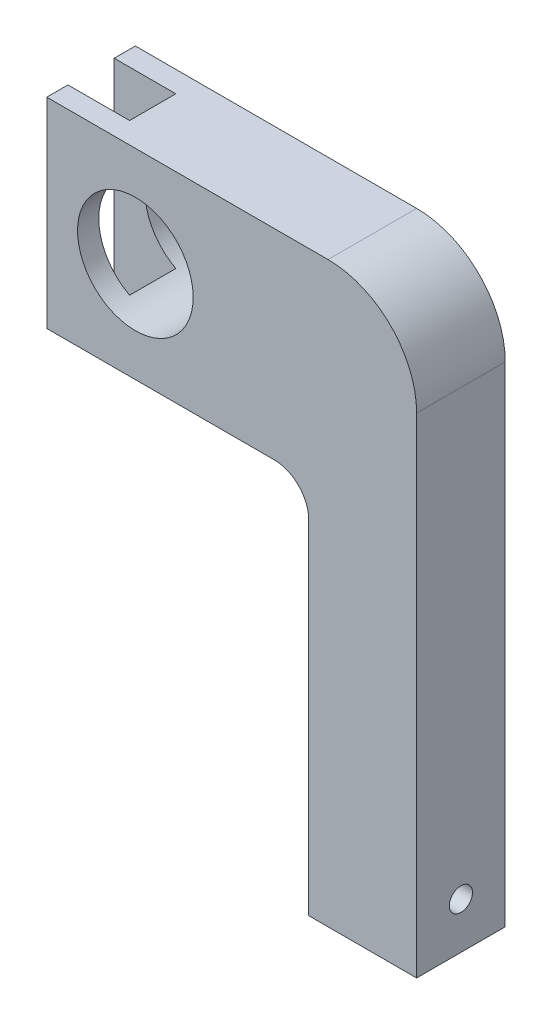
ISO-10303-21;
HEADER;
FILE_DESCRIPTION(('STEP AP214'),'2;1');
FILE_NAME('part.step','',(''),(''),'','','');
FILE_SCHEMA(('AUTOMOTIVE_DESIGN { 1 0 10303 214 1 1 1 1 }'));
ENDSEC;
DATA;
#1=APPLICATION_CONTEXT('core data for automotive mechanical design processes');
#2=APPLICATION_PROTOCOL_DEFINITION('international standard','automotive_design',2000,#1);
#3=PRODUCT_CONTEXT('',#1,'mechanical');
#4=PRODUCT('Part','Part','',(#3));
#5=PRODUCT_RELATED_PRODUCT_CATEGORY('part','',(#4));
#6=PRODUCT_DEFINITION_FORMATION('','',#4);
#7=PRODUCT_DEFINITION_CONTEXT('part definition',#1,'design');
#8=PRODUCT_DEFINITION('design','',#6,#7);
#9=PRODUCT_DEFINITION_SHAPE('','',#8);
#10=(LENGTH_UNIT() NAMED_UNIT(*) SI_UNIT(.MILLI.,.METRE.));
#11=(NAMED_UNIT(*) PLANE_ANGLE_UNIT() SI_UNIT($,.RADIAN.));
#12=(NAMED_UNIT(*) SI_UNIT($,.STERADIAN.) SOLID_ANGLE_UNIT());
#13=UNCERTAINTY_MEASURE_WITH_UNIT(LENGTH_MEASURE(1.E-05),#10,'distance_accuracy_value','');
#14=(GEOMETRIC_REPRESENTATION_CONTEXT(3) GLOBAL_UNCERTAINTY_ASSIGNED_CONTEXT((#13)) GLOBAL_UNIT_ASSIGNED_CONTEXT((#10,
#11,#12)) REPRESENTATION_CONTEXT('',''));
#15=CARTESIAN_POINT('',(0.,0.,0.));
#16=DIRECTION('',(0.,0.,1.));
#17=DIRECTION('',(1.,0.,0.));
#18=AXIS2_PLACEMENT_3D('',#15,#16,#17);
#19=CARTESIAN_POINT('',(-23.,0.,11.5));
#20=DIRECTION('',(-1.,0.,0.));
#21=DIRECTION('',(0.,0.,1.));
#22=AXIS2_PLACEMENT_3D('',#19,#20,#21);
#23=PLANE('',#22);
#24=DIRECTION('',(0.,1.,0.));
#25=VECTOR('',#24,1.);
#26=CARTESIAN_POINT('',(-23.,-37.,-6.));
#27=LINE('',#26,#25);
#28=CARTESIAN_POINT('',(-23.,-26.,-6.));
#29=VERTEX_POINT('',#28);
#30=CARTESIAN_POINT('',(-23.,26.,-6.));
#31=VERTEX_POINT('',#30);
#32=EDGE_CURVE('E195',#29,#31,#27,.T.);
#33=ORIENTED_EDGE('',*,*,#32,.T.);
#34=DIRECTION('',(0.,0.,-1.));
#35=VECTOR('',#34,1.);
#36=CARTESIAN_POINT('',(-23.,26.,11.5));
#37=LINE('',#36,#35);
#38=CARTESIAN_POINT('',(-23.,26.,-11.5));
#39=VERTEX_POINT('',#38);
#40=EDGE_CURVE('E164',#31,#39,#37,.T.);
#41=ORIENTED_EDGE('',*,*,#40,.T.);
#42=DIRECTION('',(0.,1.,0.));
#43=VECTOR('',#42,1.);
#44=CARTESIAN_POINT('',(-23.,0.,-11.5));
#45=LINE('',#44,#43);
#46=CARTESIAN_POINT('',(-23.,-26.,-11.5));
#47=VERTEX_POINT('',#46);
#48=EDGE_CURVE('E241',#47,#39,#45,.T.);
#49=ORIENTED_EDGE('',*,*,#48,.F.);
#50=DIRECTION('',(0.,0.,-1.));
#51=VECTOR('',#50,1.);
#52=CARTESIAN_POINT('',(-23.,-26.,11.5));
#53=LINE('',#52,#51);
#54=EDGE_CURVE('E262',#29,#47,#53,.T.);
#55=ORIENTED_EDGE('',*,*,#54,.F.);
#56=EDGE_LOOP('',(#33,#41,#49,#55));
#57=FACE_BOUND('',#56,.T.);
#58=ADVANCED_FACE('F41',(#57),#23,.T.);
#59=CARTESIAN_POINT('',(73.,0.,11.5));
#60=DIRECTION('',(1.,0.,0.));
#61=DIRECTION('',(0.,1.,0.));
#62=AXIS2_PLACEMENT_3D('',#59,#60,#61);
#63=PLANE('',#62);
#64=CARTESIAN_POINT('',(73.,-112.,0.));
#65=DIRECTION('',(1.,0.,0.));
#66=DIRECTION('',(0.,1.,0.));
#67=AXIS2_PLACEMENT_3D('',#64,#65,#66);
#68=CIRCLE('',#67,3.);
#69=CARTESIAN_POINT('',(73.,-109.,0.));
#70=VERTEX_POINT('',#69);
#71=EDGE_CURVE('E292',#70,#70,#68,.T.);
#72=ORIENTED_EDGE('',*,*,#71,.F.);
#73=EDGE_LOOP('',(#72));
#74=FACE_BOUND('',#73,.T.);
#75=DIRECTION('',(0.,-1.,0.));
#76=VECTOR('',#75,1.);
#77=CARTESIAN_POINT('',(73.,0.,-11.5));
#78=LINE('',#77,#76);
#79=CARTESIAN_POINT('',(73.,2.99999999999984,-11.5));
#80=VERTEX_POINT('',#79);
#81=CARTESIAN_POINT('',(73.,-124.,-11.5));
#82=VERTEX_POINT('',#81);
#83=EDGE_CURVE('E237',#80,#82,#78,.T.);
#84=ORIENTED_EDGE('',*,*,#83,.F.);
#85=DIRECTION('',(0.,0.,-1.));
#86=VECTOR('',#85,1.);
#87=CARTESIAN_POINT('',(73.,2.99999999999984,11.5));
#88=LINE('',#87,#86);
#89=CARTESIAN_POINT('',(73.,2.99999999999984,11.5));
#90=VERTEX_POINT('',#89);
#91=EDGE_CURVE('E170',#90,#80,#88,.T.);
#92=ORIENTED_EDGE('',*,*,#91,.F.);
#93=DIRECTION('',(0.,-1.,0.));
#94=VECTOR('',#93,1.);
#95=CARTESIAN_POINT('',(73.,0.,11.5));
#96=LINE('',#95,#94);
#97=CARTESIAN_POINT('',(73.,-124.,11.5));
#98=VERTEX_POINT('',#97);
#99=EDGE_CURVE('E215',#90,#98,#96,.T.);
#100=ORIENTED_EDGE('',*,*,#99,.T.);
#101=DIRECTION('',(0.,0.,-1.));
#102=VECTOR('',#101,1.);
#103=CARTESIAN_POINT('',(73.,-124.,11.5));
#104=LINE('',#103,#102);
#105=EDGE_CURVE('E235',#98,#82,#104,.T.);
#106=ORIENTED_EDGE('',*,*,#105,.T.);
#107=EDGE_LOOP('',(#84,#92,#100,#106));
#108=FACE_BOUND('',#107,.T.);
#109=ADVANCED_FACE('F319',(#74,#108),#63,.T.);
#110=CARTESIAN_POINT('',(50.,3.,11.5));
#111=DIRECTION('',(0.,0.,-1.));
#112=DIRECTION('',(-1.,0.,0.));
#113=AXIS2_PLACEMENT_3D('',#110,#111,#112);
#114=CYLINDRICAL_SURFACE('',#113,23.);
#115=CARTESIAN_POINT('',(50.,3.,-11.5));
#116=DIRECTION('',(0.,0.,1.));
#117=DIRECTION('',(1.,0.,0.));
#118=AXIS2_PLACEMENT_3D('',#115,#116,#117);
#119=CIRCLE('',#118,23.);
#120=CARTESIAN_POINT('',(49.9999999999999,26.,-11.5));
#121=VERTEX_POINT('',#120);
#122=EDGE_CURVE('E239',#80,#121,#119,.T.);
#123=ORIENTED_EDGE('',*,*,#122,.T.);
#124=DIRECTION('',(0.,0.,-1.));
#125=VECTOR('',#124,1.);
#126=CARTESIAN_POINT('',(49.9999999999999,26.,11.5));
#127=LINE('',#126,#125);
#128=CARTESIAN_POINT('',(49.9999999999999,26.,11.5));
#129=VERTEX_POINT('',#128);
#130=EDGE_CURVE('E163',#129,#121,#127,.T.);
#131=ORIENTED_EDGE('',*,*,#130,.F.);
#132=CARTESIAN_POINT('',(50.,3.,11.5));
#133=DIRECTION('',(0.,0.,1.));
#134=DIRECTION('',(1.,0.,0.));
#135=AXIS2_PLACEMENT_3D('',#132,#133,#134);
#136=CIRCLE('',#135,23.);
#137=EDGE_CURVE('E216',#90,#129,#136,.T.);
#138=ORIENTED_EDGE('',*,*,#137,.F.);
#139=ORIENTED_EDGE('',*,*,#91,.T.);
#140=EDGE_LOOP('',(#123,#131,#138,#139));
#141=FACE_BOUND('',#140,.T.);
#142=ADVANCED_FACE('F282',(#141),#114,.T.);
#143=CARTESIAN_POINT('',(0.,26.,11.5));
#144=DIRECTION('',(0.,1.,0.));
#145=DIRECTION('',(0.,0.,1.));
#146=AXIS2_PLACEMENT_3D('',#143,#144,#145);
#147=PLANE('',#146);
#148=DIRECTION('',(-1.,0.,0.));
#149=VECTOR('',#148,1.);
#150=CARTESIAN_POINT('',(-23.,26.,-6.));
#151=LINE('',#150,#149);
#152=CARTESIAN_POINT('',(-7.,26.,-6.));
#153=VERTEX_POINT('',#152);
#154=EDGE_CURVE('E149',#153,#31,#151,.T.);
#155=ORIENTED_EDGE('',*,*,#154,.F.);
#156=DIRECTION('',(0.,0.,-1.));
#157=VECTOR('',#156,1.);
#158=CARTESIAN_POINT('',(-7.,26.,-6.));
#159=LINE('',#158,#157);
#160=CARTESIAN_POINT('',(-7.,26.,6.));
#161=VERTEX_POINT('',#160);
#162=EDGE_CURVE('E158',#161,#153,#159,.T.);
#163=ORIENTED_EDGE('',*,*,#162,.F.);
#164=DIRECTION('',(1.,0.,0.));
#165=VECTOR('',#164,1.);
#166=CARTESIAN_POINT('',(-23.,26.,6.));
#167=LINE('',#166,#165);
#168=CARTESIAN_POINT('',(-23.,26.,6.));
#169=VERTEX_POINT('',#168);
#170=EDGE_CURVE('E142',#169,#161,#167,.T.);
#171=ORIENTED_EDGE('',*,*,#170,.F.);
#172=CARTESIAN_POINT('',(-23.,26.,11.5));
#173=VERTEX_POINT('',#172);
#174=EDGE_CURVE('E154',#173,#169,#37,.T.);
#175=ORIENTED_EDGE('',*,*,#174,.F.);
#176=DIRECTION('',(1.,0.,0.));
#177=VECTOR('',#176,1.);
#178=CARTESIAN_POINT('',(0.,26.,11.5));
#179=LINE('',#178,#177);
#180=EDGE_CURVE('E217',#173,#129,#179,.T.);
#181=ORIENTED_EDGE('',*,*,#180,.T.);
#182=ORIENTED_EDGE('',*,*,#130,.T.);
#183=DIRECTION('',(1.,0.,0.));
#184=VECTOR('',#183,1.);
#185=CARTESIAN_POINT('',(0.,26.,-11.5));
#186=LINE('',#185,#184);
#187=EDGE_CURVE('E244',#39,#121,#186,.T.);
#188=ORIENTED_EDGE('',*,*,#187,.F.);
#189=ORIENTED_EDGE('',*,*,#40,.F.);
#190=EDGE_LOOP('',(#155,#163,#171,#175,#181,#182,#188,#189));
#191=FACE_BOUND('',#190,.T.);
#192=ADVANCED_FACE('F153',(#191),#147,.T.);
#193=DIRECTION('',(0.,1.,0.));
#194=VECTOR('',#193,1.);
#195=CARTESIAN_POINT('',(-23.,-37.,6.));
#196=LINE('',#195,#194);
#197=CARTESIAN_POINT('',(-23.,-26.,6.));
#198=VERTEX_POINT('',#197);
#199=EDGE_CURVE('E138',#198,#169,#196,.T.);
#200=ORIENTED_EDGE('',*,*,#199,.F.);
#201=CARTESIAN_POINT('',(-23.,-26.,11.5));
#202=VERTEX_POINT('',#201);
#203=EDGE_CURVE('E166',#202,#198,#53,.T.);
#204=ORIENTED_EDGE('',*,*,#203,.F.);
#205=DIRECTION('',(0.,1.,0.));
#206=VECTOR('',#205,1.);
#207=CARTESIAN_POINT('',(-23.,0.,11.5));
#208=LINE('',#207,#206);
#209=EDGE_CURVE('E162',#202,#173,#208,.T.);
#210=ORIENTED_EDGE('',*,*,#209,.T.);
#211=ORIENTED_EDGE('',*,*,#174,.T.);
#212=EDGE_LOOP('',(#200,#204,#210,#211));
#213=FACE_BOUND('',#212,.T.);
#214=ADVANCED_FACE('F161',(#213),#23,.T.);
#215=CARTESIAN_POINT('',(0.,-26.,11.5));
#216=DIRECTION('',(0.,-1.,0.));
#217=DIRECTION('',(1.,0.,0.));
#218=AXIS2_PLACEMENT_3D('',#215,#216,#217);
#219=PLANE('',#218);
#220=DIRECTION('',(1.,0.,0.));
#221=VECTOR('',#220,1.);
#222=CARTESIAN_POINT('',(0.,-26.,-6.));
#223=LINE('',#222,#221);
#224=CARTESIAN_POINT('',(-7.,-26.,-6.));
#225=VERTEX_POINT('',#224);
#226=EDGE_CURVE('E191',#29,#225,#223,.T.);
#227=ORIENTED_EDGE('',*,*,#226,.F.);
#228=ORIENTED_EDGE('',*,*,#54,.T.);
#229=DIRECTION('',(-1.,0.,0.));
#230=VECTOR('',#229,1.);
#231=CARTESIAN_POINT('',(0.,-26.,-11.5));
#232=LINE('',#231,#230);
#233=CARTESIAN_POINT('',(36.,-26.,-11.5));
#234=VERTEX_POINT('',#233);
#235=EDGE_CURVE('E250',#234,#47,#232,.T.);
#236=ORIENTED_EDGE('',*,*,#235,.F.);
#237=DIRECTION('',(0.,0.,-1.));
#238=VECTOR('',#237,1.);
#239=CARTESIAN_POINT('',(36.,-26.,11.5));
#240=LINE('',#239,#238);
#241=CARTESIAN_POINT('',(36.,-26.,11.5));
#242=VERTEX_POINT('',#241);
#243=EDGE_CURVE('E263',#242,#234,#240,.T.);
#244=ORIENTED_EDGE('',*,*,#243,.F.);
#245=DIRECTION('',(-1.,0.,0.));
#246=VECTOR('',#245,1.);
#247=CARTESIAN_POINT('',(0.,-26.,11.5));
#248=LINE('',#247,#246);
#249=EDGE_CURVE('E222',#242,#202,#248,.T.);
#250=ORIENTED_EDGE('',*,*,#249,.T.);
#251=ORIENTED_EDGE('',*,*,#203,.T.);
#252=DIRECTION('',(-1.,0.,0.));
#253=VECTOR('',#252,1.);
#254=CARTESIAN_POINT('',(0.,-26.,6.));
#255=LINE('',#254,#253);
#256=CARTESIAN_POINT('',(-7.,-26.,6.));
#257=VERTEX_POINT('',#256);
#258=EDGE_CURVE('E144',#257,#198,#255,.T.);
#259=ORIENTED_EDGE('',*,*,#258,.F.);
#260=DIRECTION('',(0.,0.,1.));
#261=VECTOR('',#260,1.);
#262=CARTESIAN_POINT('',(-7.,-26.,11.5));
#263=LINE('',#262,#261);
#264=EDGE_CURVE('E202',#225,#257,#263,.T.);
#265=ORIENTED_EDGE('',*,*,#264,.F.);
#266=EDGE_LOOP('',(#227,#228,#236,#244,#250,#251,#259,#265));
#267=FACE_BOUND('',#266,.T.);
#268=ADVANCED_FACE('F271',(#267),#219,.T.);
#269=CARTESIAN_POINT('',(36.,-35.,11.5));
#270=DIRECTION('',(0.,0.,-1.));
#271=DIRECTION('',(-1.,0.,0.));
#272=AXIS2_PLACEMENT_3D('',#269,#270,#271);
#273=CYLINDRICAL_SURFACE('',#272,9.);
#274=CARTESIAN_POINT('',(36.,-35.,-11.5));
#275=DIRECTION('',(0.,0.,1.));
#276=DIRECTION('',(1.,0.,0.));
#277=AXIS2_PLACEMENT_3D('',#274,#275,#276);
#278=CIRCLE('',#277,9.);
#279=CARTESIAN_POINT('',(45.,-35.,-11.5));
#280=VERTEX_POINT('',#279);
#281=EDGE_CURVE('E253',#280,#234,#278,.T.);
#282=ORIENTED_EDGE('',*,*,#281,.F.);
#283=DIRECTION('',(0.,0.,-1.));
#284=VECTOR('',#283,1.);
#285=CARTESIAN_POINT('',(45.,-35.,11.5));
#286=LINE('',#285,#284);
#287=CARTESIAN_POINT('',(45.,-35.,11.5));
#288=VERTEX_POINT('',#287);
#289=EDGE_CURVE('E265',#288,#280,#286,.T.);
#290=ORIENTED_EDGE('',*,*,#289,.F.);
#291=CARTESIAN_POINT('',(36.,-35.,11.5));
#292=DIRECTION('',(0.,0.,1.));
#293=DIRECTION('',(1.,0.,0.));
#294=AXIS2_PLACEMENT_3D('',#291,#292,#293);
#295=CIRCLE('',#294,9.);
#296=EDGE_CURVE('E221',#288,#242,#295,.T.);
#297=ORIENTED_EDGE('',*,*,#296,.T.);
#298=ORIENTED_EDGE('',*,*,#243,.T.);
#299=EDGE_LOOP('',(#282,#290,#297,#298));
#300=FACE_BOUND('',#299,.T.);
#301=ADVANCED_FACE('F305',(#300),#273,.F.);
#302=CARTESIAN_POINT('',(45.,0.,11.5));
#303=DIRECTION('',(-1.,0.,0.));
#304=DIRECTION('',(0.,0.,1.));
#305=AXIS2_PLACEMENT_3D('',#302,#303,#304);
#306=PLANE('',#305);
#307=CARTESIAN_POINT('',(45.,-112.,0.));
#308=DIRECTION('',(-1.,0.,0.));
#309=DIRECTION('',(0.,0.,1.));
#310=AXIS2_PLACEMENT_3D('',#307,#308,#309);
#311=CIRCLE('',#310,3.);
#312=CARTESIAN_POINT('',(45.,-112.,3.));
#313=VERTEX_POINT('',#312);
#314=EDGE_CURVE('E44',#313,#313,#311,.T.);
#315=ORIENTED_EDGE('',*,*,#314,.F.);
#316=EDGE_LOOP('',(#315));
#317=FACE_BOUND('',#316,.T.);
#318=DIRECTION('',(0.,1.,0.));
#319=VECTOR('',#318,1.);
#320=CARTESIAN_POINT('',(45.,0.,-11.5));
#321=LINE('',#320,#319);
#322=CARTESIAN_POINT('',(45.,-124.,-11.5));
#323=VERTEX_POINT('',#322);
#324=EDGE_CURVE('E255',#323,#280,#321,.T.);
#325=ORIENTED_EDGE('',*,*,#324,.F.);
#326=DIRECTION('',(0.,0.,-1.));
#327=VECTOR('',#326,1.);
#328=CARTESIAN_POINT('',(45.,-124.,11.5));
#329=LINE('',#328,#327);
#330=CARTESIAN_POINT('',(45.,-124.,11.5));
#331=VERTEX_POINT('',#330);
#332=EDGE_CURVE('E257',#331,#323,#329,.T.);
#333=ORIENTED_EDGE('',*,*,#332,.F.);
#334=DIRECTION('',(0.,1.,0.));
#335=VECTOR('',#334,1.);
#336=CARTESIAN_POINT('',(45.,0.,11.5));
#337=LINE('',#336,#335);
#338=EDGE_CURVE('E229',#331,#288,#337,.T.);
#339=ORIENTED_EDGE('',*,*,#338,.T.);
#340=ORIENTED_EDGE('',*,*,#289,.T.);
#341=EDGE_LOOP('',(#325,#333,#339,#340));
#342=FACE_BOUND('',#341,.T.);
#343=ADVANCED_FACE('F296',(#317,#342),#306,.T.);
#344=CARTESIAN_POINT('',(0.,0.,11.5));
#345=DIRECTION('',(0.,0.,-1.));
#346=DIRECTION('',(-1.,0.,0.));
#347=AXIS2_PLACEMENT_3D('',#344,#345,#346);
#348=CYLINDRICAL_SURFACE('',#347,15.);
#349=CARTESIAN_POINT('',(0.,0.,-6.));
#350=DIRECTION('',(0.,0.,-1.));
#351=DIRECTION('',(-1.,0.,0.));
#352=AXIS2_PLACEMENT_3D('',#349,#350,#351);
#353=CIRCLE('',#352,15.);
#354=CARTESIAN_POINT('',(-7.,-13.2664991614216,-6.));
#355=VERTEX_POINT('',#354);
#356=CARTESIAN_POINT('',(-7.,13.2664991614216,-6.));
#357=VERTEX_POINT('',#356);
#358=EDGE_CURVE('E11',#355,#357,#353,.T.);
#359=ORIENTED_EDGE('',*,*,#358,.F.);
#360=DIRECTION('',(0.,0.,-1.));
#361=VECTOR('',#360,1.);
#362=CARTESIAN_POINT('',(-7.,-13.2664991614216,11.5));
#363=LINE('',#362,#361);
#364=CARTESIAN_POINT('',(-7.,-13.2664991614216,6.));
#365=VERTEX_POINT('',#364);
#366=EDGE_CURVE('E49',#365,#355,#363,.T.);
#367=ORIENTED_EDGE('',*,*,#366,.F.);
#368=CARTESIAN_POINT('',(0.,0.,6.));
#369=DIRECTION('',(0.,0.,1.));
#370=DIRECTION('',(1.,0.,0.));
#371=AXIS2_PLACEMENT_3D('',#368,#369,#370);
#372=CIRCLE('',#371,15.);
#373=CARTESIAN_POINT('',(-7.,13.2664991614216,6.));
#374=VERTEX_POINT('',#373);
#375=EDGE_CURVE('E175',#374,#365,#372,.T.);
#376=ORIENTED_EDGE('',*,*,#375,.F.);
#377=DIRECTION('',(0.,0.,-1.));
#378=VECTOR('',#377,1.);
#379=CARTESIAN_POINT('',(-7.,13.2664991614216,11.5));
#380=LINE('',#379,#378);
#381=EDGE_CURVE('E179',#357,#374,#380,.F.);
#382=ORIENTED_EDGE('',*,*,#381,.F.);
#383=EDGE_LOOP('',(#359,#367,#376,#382));
#384=FACE_BOUND('',#383,.T.);
#385=CARTESIAN_POINT('',(0.,0.,11.5));
#386=DIRECTION('',(0.,0.,1.));
#387=DIRECTION('',(1.,0.,0.));
#388=AXIS2_PLACEMENT_3D('',#385,#386,#387);
#389=CIRCLE('',#388,15.);
#390=CARTESIAN_POINT('',(15.,0.,11.5));
#391=VERTEX_POINT('',#390);
#392=EDGE_CURVE('E207',#391,#391,#389,.T.);
#393=ORIENTED_EDGE('',*,*,#392,.T.);
#394=EDGE_LOOP('',(#393));
#395=FACE_BOUND('',#394,.T.);
#396=CARTESIAN_POINT('',(0.,0.,-11.5));
#397=DIRECTION('',(0.,0.,1.));
#398=DIRECTION('',(1.,0.,0.));
#399=AXIS2_PLACEMENT_3D('',#396,#397,#398);
#400=CIRCLE('',#399,15.);
#401=CARTESIAN_POINT('',(15.,0.,-11.5));
#402=VERTEX_POINT('',#401);
#403=EDGE_CURVE('E208',#402,#402,#400,.T.);
#404=ORIENTED_EDGE('',*,*,#403,.F.);
#405=EDGE_LOOP('',(#404));
#406=FACE_BOUND('',#405,.T.);
#407=ADVANCED_FACE('F43',(#384,#395,#406),#348,.F.);
#408=CARTESIAN_POINT('',(0.,-124.,11.5));
#409=DIRECTION('',(0.,-1.,0.));
#410=DIRECTION('',(0.,0.,-1.));
#411=AXIS2_PLACEMENT_3D('',#408,#409,#410);
#412=PLANE('',#411);
#413=DIRECTION('',(-1.,0.,0.));
#414=VECTOR('',#413,1.);
#415=CARTESIAN_POINT('',(0.,-124.,-11.5));
#416=LINE('',#415,#414);
#417=EDGE_CURVE('E213',#82,#323,#416,.T.);
#418=ORIENTED_EDGE('',*,*,#417,.F.);
#419=ORIENTED_EDGE('',*,*,#105,.F.);
#420=DIRECTION('',(-1.,0.,0.));
#421=VECTOR('',#420,1.);
#422=CARTESIAN_POINT('',(0.,-124.,11.5));
#423=LINE('',#422,#421);
#424=EDGE_CURVE('E226',#98,#331,#423,.T.);
#425=ORIENTED_EDGE('',*,*,#424,.T.);
#426=ORIENTED_EDGE('',*,*,#332,.T.);
#427=EDGE_LOOP('',(#418,#419,#425,#426));
#428=FACE_BOUND('',#427,.T.);
#429=ADVANCED_FACE('F310',(#428),#412,.T.);
#430=CARTESIAN_POINT('',(0.,0.,11.5));
#431=DIRECTION('',(0.,0.,1.));
#432=DIRECTION('',(1.,0.,0.));
#433=AXIS2_PLACEMENT_3D('',#430,#431,#432);
#434=PLANE('',#433);
#435=ORIENTED_EDGE('',*,*,#392,.F.);
#436=EDGE_LOOP('',(#435));
#437=FACE_BOUND('',#436,.T.);
#438=ORIENTED_EDGE('',*,*,#99,.F.);
#439=ORIENTED_EDGE('',*,*,#137,.T.);
#440=ORIENTED_EDGE('',*,*,#180,.F.);
#441=ORIENTED_EDGE('',*,*,#209,.F.);
#442=ORIENTED_EDGE('',*,*,#249,.F.);
#443=ORIENTED_EDGE('',*,*,#296,.F.);
#444=ORIENTED_EDGE('',*,*,#338,.F.);
#445=ORIENTED_EDGE('',*,*,#424,.F.);
#446=EDGE_LOOP('',(#438,#439,#440,#441,#442,#443,#444,#445));
#447=FACE_BOUND('',#446,.T.);
#448=ADVANCED_FACE('F274',(#437,#447),#434,.T.);
#449=CARTESIAN_POINT('',(0.,0.,-11.5));
#450=DIRECTION('',(0.,0.,1.));
#451=DIRECTION('',(1.,0.,0.));
#452=AXIS2_PLACEMENT_3D('',#449,#450,#451);
#453=PLANE('',#452);
#454=ORIENTED_EDGE('',*,*,#403,.T.);
#455=EDGE_LOOP('',(#454));
#456=FACE_BOUND('',#455,.T.);
#457=ORIENTED_EDGE('',*,*,#83,.T.);
#458=ORIENTED_EDGE('',*,*,#417,.T.);
#459=ORIENTED_EDGE('',*,*,#324,.T.);
#460=ORIENTED_EDGE('',*,*,#281,.T.);
#461=ORIENTED_EDGE('',*,*,#235,.T.);
#462=ORIENTED_EDGE('',*,*,#48,.T.);
#463=ORIENTED_EDGE('',*,*,#187,.T.);
#464=ORIENTED_EDGE('',*,*,#122,.F.);
#465=EDGE_LOOP('',(#457,#458,#459,#460,#461,#462,#463,#464));
#466=FACE_BOUND('',#465,.T.);
#467=ADVANCED_FACE('F289',(#456,#466),#453,.F.);
#468=CARTESIAN_POINT('',(-7.,-37.,-6.));
#469=DIRECTION('',(1.,0.,0.));
#470=DIRECTION('',(0.,0.,-1.));
#471=AXIS2_PLACEMENT_3D('',#468,#469,#470);
#472=PLANE('',#471);
#473=ORIENTED_EDGE('',*,*,#264,.T.);
#474=DIRECTION('',(0.,1.,0.));
#475=VECTOR('',#474,1.);
#476=CARTESIAN_POINT('',(-7.,-37.,6.));
#477=LINE('',#476,#475);
#478=EDGE_CURVE('E60',#257,#365,#477,.T.);
#479=ORIENTED_EDGE('',*,*,#478,.T.);
#480=ORIENTED_EDGE('',*,*,#366,.T.);
#481=DIRECTION('',(0.,1.,0.));
#482=VECTOR('',#481,1.);
#483=CARTESIAN_POINT('',(-7.,-37.,-6.));
#484=LINE('',#483,#482);
#485=EDGE_CURVE('E181',#225,#355,#484,.T.);
#486=ORIENTED_EDGE('',*,*,#485,.F.);
#487=EDGE_LOOP('',(#473,#479,#480,#486));
#488=FACE_BOUND('',#487,.T.);
#489=ADVANCED_FACE('F185',(#488),#472,.F.);
#490=CARTESIAN_POINT('',(-23.,-37.,-6.));
#491=DIRECTION('',(0.,0.,-1.));
#492=DIRECTION('',(-1.,0.,0.));
#493=AXIS2_PLACEMENT_3D('',#490,#491,#492);
#494=PLANE('',#493);
#495=ORIENTED_EDGE('',*,*,#226,.T.);
#496=ORIENTED_EDGE('',*,*,#485,.T.);
#497=ORIENTED_EDGE('',*,*,#358,.T.);
#498=EDGE_CURVE('E193',#357,#153,#484,.T.);
#499=ORIENTED_EDGE('',*,*,#498,.T.);
#500=ORIENTED_EDGE('',*,*,#154,.T.);
#501=ORIENTED_EDGE('',*,*,#32,.F.);
#502=EDGE_LOOP('',(#495,#496,#497,#499,#500,#501));
#503=FACE_BOUND('',#502,.T.);
#504=ADVANCED_FACE('F190',(#503),#494,.F.);
#505=ORIENTED_EDGE('',*,*,#381,.T.);
#506=EDGE_CURVE('E62',#374,#161,#477,.T.);
#507=ORIENTED_EDGE('',*,*,#506,.T.);
#508=ORIENTED_EDGE('',*,*,#162,.T.);
#509=ORIENTED_EDGE('',*,*,#498,.F.);
#510=EDGE_LOOP('',(#505,#507,#508,#509));
#511=FACE_BOUND('',#510,.T.);
#512=ADVANCED_FACE('F200',(#511),#472,.F.);
#513=CARTESIAN_POINT('',(-23.,-37.,6.));
#514=DIRECTION('',(0.,0.,1.));
#515=DIRECTION('',(1.,0.,0.));
#516=AXIS2_PLACEMENT_3D('',#513,#514,#515);
#517=PLANE('',#516);
#518=ORIENTED_EDGE('',*,*,#258,.T.);
#519=ORIENTED_EDGE('',*,*,#199,.T.);
#520=ORIENTED_EDGE('',*,*,#170,.T.);
#521=ORIENTED_EDGE('',*,*,#506,.F.);
#522=ORIENTED_EDGE('',*,*,#375,.T.);
#523=ORIENTED_EDGE('',*,*,#478,.F.);
#524=EDGE_LOOP('',(#518,#519,#520,#521,#522,#523));
#525=FACE_BOUND('',#524,.T.);
#526=ADVANCED_FACE('F143',(#525),#517,.F.);
#527=CARTESIAN_POINT('',(10.,-112.,0.));
#528=DIRECTION('',(1.,0.,0.));
#529=DIRECTION('',(0.,1.,0.));
#530=AXIS2_PLACEMENT_3D('',#527,#528,#529);
#531=CYLINDRICAL_SURFACE('',#530,3.);
#532=ORIENTED_EDGE('',*,*,#314,.T.);
#533=EDGE_LOOP('',(#532));
#534=FACE_BOUND('',#533,.T.);
#535=ORIENTED_EDGE('',*,*,#71,.T.);
#536=EDGE_LOOP('',(#535));
#537=FACE_BOUND('',#536,.T.);
#538=ADVANCED_FACE('F297',(#534,#537),#531,.F.);
#539=CLOSED_SHELL('',(#58,#109,#142,#192,#214,#268,#301,#343,#407,#429,#448,#467,#489,#504,#512,
#526,#538));
#540=MANIFOLD_SOLID_BREP('B2',#539);
#541=ADVANCED_BREP_SHAPE_REPRESENTATION('',(#18,#540),#14);
#542=SHAPE_DEFINITION_REPRESENTATION(#9,#541);
ENDSEC;
END-ISO-10303-21;
